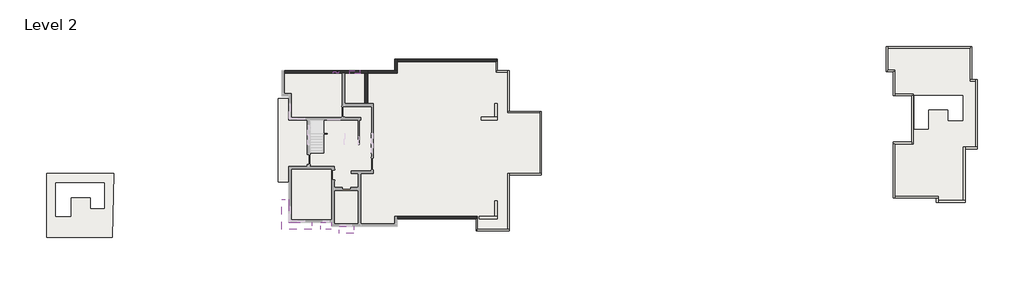
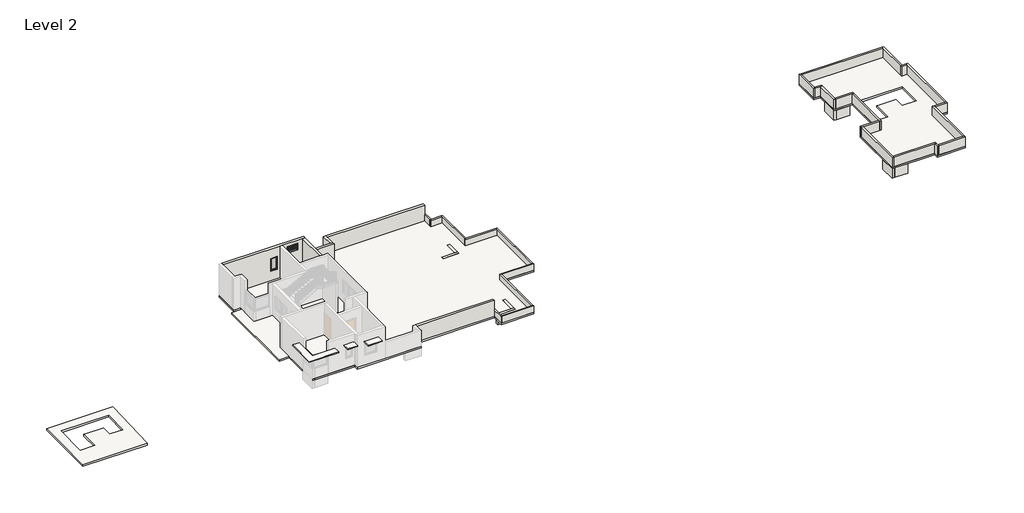
# One storey, part 2 of 5: 39 walls, 4 members, 4 slabs, 2 roofs, 1 plate, 1 window.
"""IFC4 building model written with IfcOpenShell, lengths in millimetres."""

from ifc_helpers import new_model, si_unit, frame, origin, place, context, project, spatial, polyline, outline, extrude, faceted_brep, transform, mapped, element, save
from components import member_75074519, member_86d06fe4, system_panel_glazed_1bcf12e0, window_a18e4be4

model = new_model("IFC4")

# Units and contexts
model_context = context("Model", 3, world=origin())
ifc_project = project(units=[si_unit("LENGTHUNIT", "METRE", prefix="MILLI")], contexts=[model_context])

# Site, building, storey
site = spatial("IfcSite", under=ifc_project)
building = spatial("IfcBuilding", under=site)
storey = spatial("IfcBuildingStorey", under=building, Name="Level 2", Elevation=3048.0)

# Members
placement = place(None, origin())
member_shape = member_75074519(model_context)
element("IfcMember", 1, ObjectType="Rectangular Mullion : 2.5\" x 5\" rectangular", at=placement, inside=storey, context=model_context, shape_type="MappedRepresentation", body=[
    mapped(member_shape, transform((-38334.7146233, 19736.4864709, 3962.4), x_axis=(1.0, 0.0, 0.0), y_axis=(0.0, -1.0, 0.0), z_axis=(0.0, 0.0, -1.0))),
])
element("IfcMember", 2, ObjectType="Rectangular Mullion : 2.5\" x 5\" rectangular", at=placement, inside=storey, context=model_context, shape_type="MappedRepresentation", body=[
    mapped(member_shape, transform((-38944.3146233, 19736.4864709, 5181.6), x_axis=(-1.0, 0.0, 0.0), y_axis=(0.0, -1.0, 0.0), z_axis=(0.0, 0.0, 1.0))),
])
member_2_shape = member_86d06fe4(model_context)
element("IfcMember", 3, ObjectType="Rectangular Mullion : 2.5\" x 5\" rectangular", at=placement, inside=storey, context=model_context, shape_type="MappedRepresentation", body=[
    mapped(member_2_shape, transform((-38398.2146233, 19736.4864709, 5181.6), x_axis=(0.0, 0.0, 1.0), y_axis=(0.0, -1.0, 0.0), z_axis=(1.0, 0.0, 0.0))),
])
element("IfcMember", 4, ObjectType="Rectangular Mullion : 2.5\" x 5\" rectangular", at=placement, inside=storey, context=model_context, shape_type="MappedRepresentation", body=[
    mapped(member_2_shape, transform((-38880.8146233, 19736.4864709, 3962.4), x_axis=(0.0, 0.0, -1.0), y_axis=(0.0, -1.0, 0.0), z_axis=(-1.0, 0.0, 0.0))),
])

# Plate
system_panel_glazed_shape = system_panel_glazed_1bcf12e0(model_context)
element("IfcPlate", 5, ObjectType="System Panel : Glazed", at=placement, inside=storey, context=model_context, shape_type="MappedRepresentation", body=[
    mapped(system_panel_glazed_shape, transform((-38639.5146233, 19736.4864709, 4025.9), x_axis=(1.0, 0.0, 0.0), y_axis=(0.0, 1.0, 0.0), z_axis=(0.0, 0.0, 1.0))),
])

# Roofs
element("IfcRoof", 6, ObjectType="ROOF 6\"", at=placement, inside=storey, context=model_context, shape_type="SweptSolid", body=[
    extrude(outline(polyline([(11387.9100959, 17645.0480703), (11387.9100959, 19778.6480703), (10778.3100959, 19778.6480703), (10778.3100959, 22064.6480703), (18474.5100959, 22064.6480703), (18474.5100959, 19092.8480703), (18969.8100959, 19092.8480703), (18969.8100959, 12844.4480703), (17864.9100959, 12844.4480703), (17864.9100959, 8043.769664), (15274.1100959, 8043.769664), (15274.1100959, 8424.8480703), (11387.9100959, 8424.8480703), (11387.9100959, 13454.0480703), (13064.3100959, 13454.0480703), (13064.3100959, 17645.0480703), (11387.9100959, 17645.0480703)]), holes=[polyline([(17636.3100959, 17645.0480703), (13292.9100959, 17645.0480703), (13292.9100959, 14647.8480703), (14562.9100959, 14647.8480703), (14562.9100959, 16375.0480703), (16366.3100959, 16375.0480703), (16366.3100959, 15409.8480703), (17636.3100959, 15409.8480703), (17636.3100959, 17645.0480703)])]), frame((0.0, 0.0, 3048.0), z_axis=(0.0, 0.0, 1.0), x_axis=(1.0, 0.0, 0.0)), (0.0, 0.0, 1.0), 152.4),
])
element("IfcRoof", 7, ObjectType="ROOF 6\"", at=placement, inside=storey, context=model_context, shape_type="SweptSolid", body=[
    extrude(outline(polyline([(-58617.9939273, 10640.5199577), (-58763.0300618, 4887.4199577), (-64652.8636189, 4887.4199577), (-64652.8636189, 10640.5199577), (-58617.9939273, 10640.5199577)]), holes=[polyline([(-62493.8636189, 6754.3199577), (-62493.8636189, 8481.5199577), (-60690.4636189, 8481.5199577), (-60690.4636189, 7516.3199577), (-59471.2636189, 7516.3199577), (-59471.2636189, 9802.3199577), (-63814.6636189, 9802.3199577), (-63814.6636189, 6754.3199577), (-62493.8636189, 6754.3199577)])]), frame((0.0, 0.0, 3048.0), z_axis=(0.0, 0.0, 1.0), x_axis=(1.0, 0.0, 0.0)), (0.0, 0.0, 1.0), 152.4),
])

# Slabs
element("IfcSlab", 8, ObjectType="FLOOR 6\"", at=placement, inside=storey, context=model_context, shape_type="SweptSolid", body=[
    extrude(outline(polyline([(-43821.1146233, 17357.3026655), (-42906.7146233, 17357.3026655), (-42906.7146233, 17590.1864709), (-43516.3146233, 17590.1864709), (-43516.3146233, 19876.1864709), (-33382.215517, 19876.1864709), (-33382.215517, 20942.9864709), (-24161.5146233, 20942.9864709), (-24161.5146233, 19876.1864709), (-23094.7146233, 19876.1864709), (-23094.7146233, 16218.5864709), (-20199.1146233, 16218.5864709), (-20199.1146233, 10503.5864709), (-23094.7146233, 10503.5864709), (-23094.7146233, 5474.3864709), (-26066.5146233, 5474.3864709), (-26066.5146233, 6541.1864709), (-33153.1146233, 6541.1864709), (-33153.1146233, 5855.3080647), (-39020.5146233, 5855.3080647), (-39020.5146233, 6236.3864709), (-42906.7146233, 6236.3864709), (-42906.7146233, 9893.9864709), (-43821.1146233, 9893.9864709), (-43821.1146233, 17357.3026655)])), frame((0.0, 0.0, 2895.6), z_axis=(0.0, 0.0, 1.0), x_axis=(1.0, 0.0, 0.0)), (0.0, 0.0, 1.0), 152.4),
])
element("IfcSlab", 9, ObjectType="Generic - 12\"", at=placement, inside=storey, context=model_context, shape_type="SweptSolid", body=[
    extrude(outline(polyline([(-43516.3146234, 8293.7864709), (-42906.7146233, 8293.7864709), (-42906.7146233, 6236.3864709), (-40849.3146233, 6236.3864709), (-40849.3146233, 5626.7864709), (-43516.3146234, 5626.7864709), (-43516.3146234, 8293.7864709)])), frame((0.0, 0.0, 5257.8), z_axis=(0.0, 0.0, 1.0), x_axis=(1.0, 0.0, 0.0)), (0.0, 0.0, 1.0), 76.2),
])
element("IfcSlab", 10, ObjectType="Generic - 12\"", at=placement, inside=storey, context=model_context, shape_type="SweptSolid", body=[
    extrude(outline(polyline([(-40011.1146233, 5626.7864709), (-40011.1146233, 6236.3864709), (-39096.7146233, 6236.3864709), (-39096.7146233, 5626.7864709), (-40011.1146233, 5626.7864709)])), frame((0.0, 0.0, 5257.8), z_axis=(0.0, 0.0, 1.0), x_axis=(1.0, 0.0, 0.0)), (0.0, 0.0, 1.0), 76.2),
])
element("IfcSlab", 11, ObjectType="Generic - 12\"", at=placement, inside=storey, context=model_context, shape_type="SweptSolid", body=[
    extrude(outline(polyline([(-38372.8146233, 5245.7080647), (-38372.8146233, 5855.3080647), (-37077.4146233, 5855.3080647), (-37077.4146233, 5245.7080647), (-38372.8146233, 5245.7080647)])), frame((0.0, 0.0, 5257.8), z_axis=(0.0, 0.0, 1.0), x_axis=(1.0, 0.0, 0.0)), (0.0, 0.0, 1.0), 76.2),
])

# Walls
element("IfcWall", 12, at=placement, inside=storey, context=model_context, shape_type="Brep", body=[
    faceted_brep([(-35820.1146233, 19647.5864709, 3048.0), (-33153.615517, 19647.5864709, 3048.0), (-33153.615517, 19647.5864709, 4572.0), (-35820.1146233, 19647.5864709, 4572.0), (-35820.1146233, 19876.1864709, 3048.0), (-35820.1146233, 19876.1864709, 4572.0), (-33382.215517, 19876.1864709, 4572.0), (-33153.615517, 19876.1864709, 4572.0), (-33153.615517, 19876.1864709, 3048.0), (-33382.215517, 19876.1864709, 3048.0)], [[[0, 1, 2, 3]], [[4, 5, 6, 7, 8, 9]], [[1, 0, 4, 9, 8]], [[3, 2, 7, 6, 5]], [[2, 1, 8, 7]], [[0, 3, 5, 4]]]),
])
element("IfcWall", 13, at=placement, inside=storey, context=model_context, shape_type="Brep", body=[
    faceted_brep([(-33153.615517, 19876.1864709, 3048.0), (-33153.615517, 20714.3864709, 3048.0), (-33153.615517, 20942.9864709, 3048.0), (-33153.615517, 20942.9864709, 4572.0), (-33153.615517, 20714.3864709, 4572.0), (-33153.615517, 19876.1864709, 4572.0), (-33382.215517, 19876.1864709, 3048.0), (-33382.215517, 19876.1864709, 4572.0), (-33382.215517, 20942.9864709, 4572.0), (-33382.215517, 20942.9864709, 3048.0)], [[[0, 1, 2, 3, 4, 5]], [[6, 7, 8, 9]], [[2, 1, 0, 6, 9]], [[5, 4, 3, 8, 7]], [[0, 5, 7, 6]], [[3, 2, 9, 8]]]),
])
element("IfcWall", 14, at=placement, inside=storey, context=model_context, shape_type="Brep", body=[
    faceted_brep([(-33153.615517, 20714.3864709, 3048.0), (-24275.8146233, 20714.3864709, 3048.0), (-24275.8146233, 20714.3864709, 4572.0), (-33153.615517, 20714.3864709, 4572.0), (-33153.615517, 20942.9864709, 3048.0), (-33153.615517, 20942.9864709, 4572.0), (-24275.8146233, 20942.9864709, 4572.0), (-24275.8146233, 20942.9864709, 3657.6), (-24275.8146233, 20942.9864709, 3048.0)], [[[0, 1, 2, 3]], [[4, 5, 6, 7, 8]], [[1, 0, 4, 8]], [[3, 2, 6, 5]], [[0, 3, 5, 4]], [[2, 1, 8, 7, 6]]]),
])
element("IfcWall", 15, at=placement, inside=storey, context=model_context, shape_type="Brep", body=[
    faceted_brep([(-33153.1146233, 6541.1864709, 3048.0), (-26066.5146233, 6541.1864709, 3048.0), (-26066.5146233, 6541.1864709, 4572.0), (-33153.1146233, 6541.1864709, 4572.0), (-33153.1146233, 6769.7864709, 3048.0), (-33153.1146233, 6769.7864709, 4572.0), (-26066.5146233, 6769.7864709, 4572.0), (-26066.5146233, 6769.7864709, 3657.6), (-26066.5146233, 6769.7864709, 3048.0)], [[[0, 1, 2, 3]], [[4, 5, 6, 7, 8]], [[1, 0, 4, 8]], [[3, 2, 6, 5]], [[0, 3, 5, 4]], [[2, 1, 8, 7, 6]]]),
])
element("IfcWall", 16, at=placement, inside=storey, context=model_context, shape_type="Brep", body=[
    faceted_brep([(-26066.5146233, 6769.7864709, 3048.0), (-26066.5146233, 6541.1864709, 3048.0), (-26066.5146233, 5474.3864709, 3048.0), (-26066.5146233, 5474.3864709, 3657.6), (-26066.5146233, 6769.7864709, 3657.6), (-25952.2146233, 6769.7864709, 3048.0), (-25952.2146233, 6769.7864709, 3657.6), (-25952.2146233, 5588.6864709, 3657.6), (-25952.2146233, 5474.3864709, 3657.6), (-25952.2146233, 5474.3864709, 3048.0), (-25952.2146233, 5588.6864709, 3048.0)], [[[0, 1, 2, 3, 4]], [[5, 6, 7, 8, 9, 10]], [[2, 1, 0, 5, 10, 9]], [[4, 3, 8, 7, 6]], [[0, 4, 6, 5]], [[3, 2, 9, 8]]]),
])
element("IfcWall", 17, at=placement, inside=storey, context=model_context, shape_type="Brep", body=[
    faceted_brep([(-25952.2146233, 5474.3864709, 3048.0), (-23094.7146233, 5474.3864709, 3048.0), (-23094.7146233, 5474.3864709, 3657.6), (-25952.2146233, 5474.3864709, 3657.6), (-25952.2146233, 5588.6864709, 3048.0), (-25952.2146233, 5588.6864709, 3657.6), (-23209.0146233, 5588.6864709, 3657.6), (-23094.7146233, 5588.6864709, 3657.6), (-23094.7146233, 5588.6864709, 3048.0), (-23209.0146233, 5588.6864709, 3048.0)], [[[0, 1, 2, 3]], [[4, 5, 6, 7, 8, 9]], [[1, 0, 4, 9, 8]], [[3, 2, 7, 6, 5]], [[0, 3, 5, 4]], [[2, 1, 8, 7]]]),
])
element("IfcWall", 18, at=placement, inside=storey, context=model_context, shape_type="Brep", body=[
    faceted_brep([(-23094.7146233, 5588.6864709, 3048.0), (-23094.7146233, 10503.5864709, 3048.0), (-23094.7146233, 10617.8864709, 3048.0), (-23094.7146233, 10617.8864709, 3657.6), (-23094.7146233, 10503.5864709, 3657.6), (-23094.7146233, 5588.6864709, 3657.6), (-23209.0146233, 5588.6864709, 3048.0), (-23209.0146233, 5588.6864709, 3657.6), (-23209.0146233, 10617.8864709, 3657.6), (-23209.0146233, 10617.8864709, 3048.0)], [[[0, 1, 2, 3, 4, 5]], [[6, 7, 8, 9]], [[2, 1, 0, 6, 9]], [[5, 4, 3, 8, 7]], [[0, 5, 7, 6]], [[3, 2, 9, 8]]]),
])
element("IfcWall", 19, at=placement, inside=storey, context=model_context, shape_type="Brep", body=[
    faceted_brep([(-23094.7146233, 10503.5864709, 3048.0), (-20199.1146233, 10503.5864709, 3048.0), (-20199.1146233, 10503.5864709, 3657.6), (-23094.7146233, 10503.5864709, 3657.6), (-23094.7146233, 10617.8864709, 3048.0), (-23094.7146233, 10617.8864709, 3657.6), (-20313.4146233, 10617.8864709, 3657.6), (-20199.1146233, 10617.8864709, 3657.6), (-20199.1146233, 10617.8864709, 3048.0), (-20313.4146233, 10617.8864709, 3048.0)], [[[0, 1, 2, 3]], [[4, 5, 6, 7, 8, 9]], [[1, 0, 4, 9, 8]], [[3, 2, 7, 6, 5]], [[0, 3, 5, 4]], [[2, 1, 8, 7]]]),
])
element("IfcWall", 20, at=placement, inside=storey, context=model_context, shape_type="Brep", body=[
    faceted_brep([(-20199.1146233, 10617.8864709, 3048.0), (-20199.1146233, 16218.5864709, 3048.0), (-20199.1146233, 16218.5864709, 3657.6), (-20199.1146233, 10617.8864709, 3657.6), (-20313.4146233, 10617.8864709, 3048.0), (-20313.4146233, 10617.8864709, 3657.6), (-20313.4146233, 16104.2864709, 3657.6), (-20313.4146233, 16218.5864709, 3657.6), (-20313.4146233, 16218.5864709, 3048.0), (-20313.4146233, 16104.2864709, 3048.0)], [[[0, 1, 2, 3]], [[4, 5, 6, 7, 8, 9]], [[1, 0, 4, 9, 8]], [[3, 2, 7, 6, 5]], [[0, 3, 5, 4]], [[2, 1, 8, 7]]]),
])
element("IfcWall", 21, at=placement, inside=storey, context=model_context, shape_type="Brep", body=[
    faceted_brep([(-20313.4146233, 16218.5864709, 3048.0), (-23094.7146233, 16218.5864709, 3048.0), (-23209.0146233, 16218.5864709, 3048.0), (-23209.0146233, 16218.5864709, 3657.6), (-23094.7146233, 16218.5864709, 3657.6), (-20313.4146233, 16218.5864709, 3657.6), (-20313.4146233, 16104.2864709, 3048.0), (-20313.4146233, 16104.2864709, 3657.6), (-23209.0146233, 16104.2864709, 3657.6), (-23209.0146233, 16104.2864709, 3048.0)], [[[0, 1, 2, 3, 4, 5]], [[6, 7, 8, 9]], [[2, 1, 0, 6, 9]], [[5, 4, 3, 8, 7]], [[0, 5, 7, 6]], [[3, 2, 9, 8]]]),
])
element("IfcWall", 22, at=placement, inside=storey, context=model_context, shape_type="Brep", body=[
    faceted_brep([(-23094.7146233, 16218.5864709, 3048.0), (-23094.7146233, 19876.1864709, 3048.0), (-23094.7146233, 19876.1864709, 3657.6), (-23094.7146233, 16218.5864709, 3657.6), (-23209.0146233, 16218.5864709, 3048.0), (-23209.0146233, 16218.5864709, 3657.6), (-23209.0146233, 19761.8864709, 3657.6), (-23209.0146233, 19876.1864709, 3657.6), (-23209.0146233, 19876.1864709, 3048.0), (-23209.0146233, 19761.8864709, 3048.0)], [[[0, 1, 2, 3]], [[4, 5, 6, 7, 8, 9]], [[1, 0, 4, 9, 8]], [[3, 2, 7, 6, 5]], [[0, 3, 5, 4]], [[2, 1, 8, 7]]]),
])
element("IfcWall", 23, at=placement, inside=storey, context=model_context, shape_type="Brep", body=[
    faceted_brep([(-23209.0146233, 19876.1864709, 3048.0), (-24161.5146233, 19876.1864709, 3048.0), (-24275.8146233, 19876.1864709, 3048.0), (-24275.8146233, 19876.1864709, 3657.6), (-24161.5146233, 19876.1864709, 3657.6), (-23209.0146233, 19876.1864709, 3657.6), (-23209.0146233, 19761.8864709, 3048.0), (-23209.0146233, 19761.8864709, 3657.6), (-24275.8146233, 19761.8864709, 3657.6), (-24275.8146233, 19761.8864709, 3048.0)], [[[0, 1, 2, 3, 4, 5]], [[6, 7, 8, 9]], [[2, 1, 0, 6, 9]], [[5, 4, 3, 8, 7]], [[0, 5, 7, 6]], [[3, 2, 9, 8]]]),
])
element("IfcWall", 24, at=placement, inside=storey, context=model_context, shape_type="Brep", body=[
    faceted_brep([(-24161.5146233, 19876.1864709, 3048.0), (-24161.5146233, 20942.9864709, 3048.0), (-24161.5146233, 20942.9864709, 3657.6), (-24161.5146233, 19876.1864709, 3657.6), (-24275.8146233, 19876.1864709, 3048.0), (-24275.8146233, 19876.1864709, 3657.6), (-24275.8146233, 20942.9864709, 3657.6), (-24275.8146233, 20942.9864709, 3048.0), (-24275.8146233, 20714.3864709, 3048.0)], [[[0, 1, 2, 3]], [[4, 5, 6, 7, 8]], [[1, 0, 4, 8, 7]], [[3, 2, 6, 5]], [[0, 3, 5, 4]], [[2, 1, 7, 6]]]),
])
element("IfcWall", 25, ObjectType="PARAPET WALL", at=placement, inside=storey, context=model_context, shape_type="Brep", body=[
    faceted_brep([(10778.3100959, 22064.6480703, 3200.4), (10778.3100959, 19778.6480703, 3200.4), (10778.3100959, 19778.6480703, 4114.8), (10778.3100959, 22064.6480703, 4114.8), (10930.7100959, 22064.6480703, 3200.4), (10930.7100959, 22064.6480703, 4114.8), (10930.7100959, 21912.2480703, 4114.8), (10930.7100959, 19931.0480703, 4114.8), (10930.7100959, 19778.6480703, 4114.8), (10930.7100959, 19778.6480703, 3200.4), (10930.7100959, 19931.0480703, 3200.4), (10930.7100959, 21912.2480703, 3200.4)], [[[0, 1, 2, 3]], [[4, 5, 6, 7, 8, 9, 10, 11]], [[1, 0, 4, 11, 10, 9]], [[3, 2, 8, 7, 6, 5]], [[2, 1, 9, 8]], [[0, 3, 5, 4]]]),
])
element("IfcWall", 26, ObjectType="PARAPET WALL", at=placement, inside=storey, context=model_context, shape_type="Brep", body=[
    faceted_brep([(10930.7100959, 19778.6480703, 3200.4), (11387.9100959, 19778.6480703, 3200.4), (11540.3100959, 19778.6480703, 3200.4), (11540.3100959, 19778.6480703, 4114.8), (11387.9100959, 19778.6480703, 4114.8), (10930.7100959, 19778.6480703, 4114.8), (10930.7100959, 19931.0480703, 3200.4), (10930.7100959, 19931.0480703, 4114.8), (11540.3100959, 19931.0480703, 4114.8), (11540.3100959, 19931.0480703, 3200.4)], [[[0, 1, 2, 3, 4, 5]], [[6, 7, 8, 9]], [[2, 1, 0, 6, 9]], [[5, 4, 3, 8, 7]], [[0, 5, 7, 6]], [[3, 2, 9, 8]]]),
])
element("IfcWall", 27, ObjectType="PARAPET WALL", at=placement, inside=storey, context=model_context, shape_type="Brep", body=[
    faceted_brep([(11387.9100959, 19778.6480703, 3200.4), (11387.9100959, 17645.0480703, 3200.4), (11387.9100959, 17645.0480703, 4114.8), (11387.9100959, 19778.6480703, 4114.8), (11540.3100959, 19778.6480703, 3200.4), (11540.3100959, 19778.6480703, 4114.8), (11540.3100959, 17797.4480703, 4114.8), (11540.3100959, 17645.0480703, 4114.8), (11540.3100959, 17645.0480703, 3200.4), (11540.3100959, 17797.4480703, 3200.4)], [[[0, 1, 2, 3]], [[4, 5, 6, 7, 8, 9]], [[1, 0, 4, 9, 8]], [[3, 2, 7, 6, 5]], [[0, 3, 5, 4]], [[2, 1, 8, 7]]]),
])
element("IfcWall", 28, ObjectType="PARAPET WALL", at=placement, inside=storey, context=model_context, shape_type="Brep", body=[
    faceted_brep([(11540.3100959, 17645.0480703, 3200.4), (13064.3100959, 17645.0480703, 3200.4), (13216.7100959, 17645.0480703, 3200.4), (13216.7100959, 17645.0480703, 4114.8), (13064.3100959, 17645.0480703, 4114.8), (11540.3100959, 17645.0480703, 4114.8), (11540.3100959, 17797.4480703, 3200.4), (11540.3100959, 17797.4480703, 4114.8), (13216.7100959, 17797.4480703, 4114.8), (13216.7100959, 17797.4480703, 3200.4)], [[[0, 1, 2, 3, 4, 5]], [[6, 7, 8, 9]], [[2, 1, 0, 6, 9]], [[5, 4, 3, 8, 7]], [[0, 5, 7, 6]], [[3, 2, 9, 8]]]),
])
element("IfcWall", 29, ObjectType="PARAPET WALL", at=placement, inside=storey, context=model_context, shape_type="Brep", body=[
    faceted_brep([(13064.3100959, 17645.0480703, 3200.4), (13064.3100959, 13454.0480703, 3200.4), (13064.3100959, 13301.6480703, 3200.4), (13064.3100959, 13301.6480703, 4114.8), (13064.3100959, 13454.0480703, 4114.8), (13064.3100959, 17645.0480703, 4114.8), (13216.7100959, 17645.0480703, 3200.4), (13216.7100959, 17645.0480703, 4114.8), (13216.7100959, 13301.6480703, 4114.8), (13216.7100959, 13301.6480703, 3200.4)], [[[0, 1, 2, 3, 4, 5]], [[6, 7, 8, 9]], [[2, 1, 0, 6, 9]], [[5, 4, 3, 8, 7]], [[0, 5, 7, 6]], [[3, 2, 9, 8]]]),
])
element("IfcWall", 30, ObjectType="PARAPET WALL", at=placement, inside=storey, context=model_context, shape_type="Brep", body=[
    faceted_brep([(13064.3100959, 13454.0480703, 3200.4), (11387.9100959, 13454.0480703, 3200.4), (11387.9100959, 13454.0480703, 4114.8), (13064.3100959, 13454.0480703, 4114.8), (13064.3100959, 13301.6480703, 3200.4), (13064.3100959, 13301.6480703, 4114.8), (11540.3100959, 13301.6480703, 4114.8), (11387.9100959, 13301.6480703, 4114.8), (11387.9100959, 13301.6480703, 3200.4), (11540.3100959, 13301.6480703, 3200.4)], [[[0, 1, 2, 3]], [[4, 5, 6, 7, 8, 9]], [[1, 0, 4, 9, 8]], [[3, 2, 7, 6, 5]], [[0, 3, 5, 4]], [[2, 1, 8, 7]]]),
])
element("IfcWall", 31, ObjectType="PARAPET WALL", at=placement, inside=storey, context=model_context, shape_type="Brep", body=[
    faceted_brep([(11387.9100959, 13301.6480703, 3200.4), (11387.9100959, 8424.8480703, 3200.4), (11387.9100959, 8424.8480703, 4114.8), (11387.9100959, 13301.6480703, 4114.8), (11540.3100959, 13301.6480703, 3200.4), (11540.3100959, 13301.6480703, 4114.8), (11540.3100959, 8577.2480703, 4114.8), (11540.3100959, 8424.8480703, 4114.8), (11540.3100959, 8424.8480703, 3200.4), (11540.3100959, 8577.2480703, 3200.4)], [[[0, 1, 2, 3]], [[4, 5, 6, 7, 8, 9]], [[1, 0, 4, 9, 8]], [[3, 2, 7, 6, 5]], [[0, 3, 5, 4]], [[2, 1, 8, 7]]]),
])
element("IfcWall", 32, ObjectType="PARAPET WALL", at=placement, inside=storey, context=model_context, shape_type="Brep", body=[
    faceted_brep([(11540.3100959, 8424.8480703, 3200.4), (15274.1100959, 8424.8480703, 3200.4), (15426.5100959, 8424.8480703, 3200.4), (15426.5100959, 8424.8480703, 4114.8), (15274.1100959, 8424.8480703, 4114.8), (11540.3100959, 8424.8480703, 4114.8), (11540.3100959, 8577.2480703, 3200.4), (11540.3100959, 8577.2480703, 4114.8), (15426.5100959, 8577.2480703, 4114.8), (15426.5100959, 8577.2480703, 3200.4)], [[[0, 1, 2, 3, 4, 5]], [[6, 7, 8, 9]], [[2, 1, 0, 6, 9]], [[5, 4, 3, 8, 7]], [[0, 5, 7, 6]], [[3, 2, 9, 8]]]),
])
element("IfcWall", 33, ObjectType="PARAPET WALL", at=placement, inside=storey, context=model_context, shape_type="Brep", body=[
    faceted_brep([(15274.1100959, 8424.8480703, 3200.4), (15274.1100959, 8043.769664, 3200.4), (15274.1100959, 8043.769664, 4114.8), (15274.1100959, 8424.8480703, 4114.8), (15426.5100959, 8424.8480703, 3200.4), (15426.5100959, 8424.8480703, 4114.8), (15426.5100959, 8196.169664, 4114.8), (15426.5100959, 8043.769664, 4114.8), (15426.5100959, 8043.769664, 3200.4), (15426.5100959, 8196.169664, 3200.4)], [[[0, 1, 2, 3]], [[4, 5, 6, 7, 8, 9]], [[1, 0, 4, 9, 8]], [[3, 2, 7, 6, 5]], [[0, 3, 5, 4]], [[2, 1, 8, 7]]]),
])
element("IfcWall", 34, ObjectType="PARAPET WALL", at=placement, inside=storey, context=model_context, shape_type="Brep", body=[
    faceted_brep([(15426.5100959, 8043.769664, 3200.4), (17864.9100959, 8043.769664, 3200.4), (17864.9100959, 8043.769664, 4114.8), (15426.5100959, 8043.769664, 4114.8), (15426.5100959, 8196.169664, 3200.4), (15426.5100959, 8196.169664, 4114.8), (17712.5100959, 8196.169664, 4114.8), (17864.9100959, 8196.169664, 4114.8), (17864.9100959, 8196.169664, 3200.4), (17712.5100959, 8196.169664, 3200.4)], [[[0, 1, 2, 3]], [[4, 5, 6, 7, 8, 9]], [[1, 0, 4, 9, 8]], [[3, 2, 7, 6, 5]], [[0, 3, 5, 4]], [[2, 1, 8, 7]]]),
])
element("IfcWall", 35, ObjectType="PARAPET WALL", at=placement, inside=storey, context=model_context, shape_type="Brep", body=[
    faceted_brep([(17864.9100959, 8196.169664, 3200.4), (17864.9100959, 12844.4480703, 3200.4), (17864.9100959, 12996.8480703, 3200.4), (17864.9100959, 12996.8480703, 4114.8), (17864.9100959, 12844.4480703, 4114.8), (17864.9100959, 8196.169664, 4114.8), (17712.5100959, 8196.169664, 3200.4), (17712.5100959, 8196.169664, 4114.8), (17712.5100959, 12996.8480703, 4114.8), (17712.5100959, 12996.8480703, 3200.4)], [[[0, 1, 2, 3, 4, 5]], [[6, 7, 8, 9]], [[2, 1, 0, 6, 9]], [[5, 4, 3, 8, 7]], [[0, 5, 7, 6]], [[3, 2, 9, 8]]]),
])
element("IfcWall", 36, ObjectType="PARAPET WALL", at=placement, inside=storey, context=model_context, shape_type="Brep", body=[
    faceted_brep([(17864.9100959, 12844.4480703, 3200.4), (18969.8100959, 12844.4480703, 3200.4), (18969.8100959, 12844.4480703, 4114.8), (17864.9100959, 12844.4480703, 4114.8), (17864.9100959, 12996.8480703, 3200.4), (17864.9100959, 12996.8480703, 4114.8), (18817.4100959, 12996.8480703, 4114.8), (18969.8100959, 12996.8480703, 4114.8), (18969.8100959, 12996.8480703, 3200.4), (18817.4100959, 12996.8480703, 3200.4)], [[[0, 1, 2, 3]], [[4, 5, 6, 7, 8, 9]], [[1, 0, 4, 9, 8]], [[3, 2, 7, 6, 5]], [[0, 3, 5, 4]], [[2, 1, 8, 7]]]),
])
element("IfcWall", 37, ObjectType="PARAPET WALL", at=placement, inside=storey, context=model_context, shape_type="Brep", body=[
    faceted_brep([(18969.8100959, 12996.8480703, 3200.4), (18969.8100959, 19092.8480703, 3200.4), (18969.8100959, 19092.8480703, 4114.8), (18969.8100959, 12996.8480703, 4114.8), (18817.4100959, 12996.8480703, 3200.4), (18817.4100959, 12996.8480703, 4114.8), (18817.4100959, 18940.4480703, 4114.8), (18817.4100959, 19092.8480703, 4114.8), (18817.4100959, 19092.8480703, 3200.4), (18817.4100959, 18940.4480703, 3200.4)], [[[0, 1, 2, 3]], [[4, 5, 6, 7, 8, 9]], [[1, 0, 4, 9, 8]], [[3, 2, 7, 6, 5]], [[0, 3, 5, 4]], [[2, 1, 8, 7]]]),
])
element("IfcWall", 38, ObjectType="PARAPET WALL", at=placement, inside=storey, context=model_context, shape_type="Brep", body=[
    faceted_brep([(18817.4100959, 19092.8480703, 3200.4), (18474.5100959, 19092.8480703, 3200.4), (18322.1100959, 19092.8480703, 3200.4), (18322.1100959, 19092.8480703, 4114.8), (18474.5100959, 19092.8480703, 4114.8), (18817.4100959, 19092.8480703, 4114.8), (18817.4100959, 18940.4480703, 3200.4), (18817.4100959, 18940.4480703, 4114.8), (18322.1100959, 18940.4480703, 4114.8), (18322.1100959, 18940.4480703, 3200.4)], [[[0, 1, 2, 3, 4, 5]], [[6, 7, 8, 9]], [[2, 1, 0, 6, 9]], [[5, 4, 3, 8, 7]], [[0, 5, 7, 6]], [[3, 2, 9, 8]]]),
])
element("IfcWall", 39, ObjectType="PARAPET WALL", at=placement, inside=storey, context=model_context, shape_type="Brep", body=[
    faceted_brep([(18474.5100959, 19092.8480703, 3200.4), (18474.5100959, 22064.6480703, 3200.4), (18474.5100959, 22064.6480703, 4114.8), (18474.5100959, 19092.8480703, 4114.8), (18322.1100959, 19092.8480703, 3200.4), (18322.1100959, 19092.8480703, 4114.8), (18322.1100959, 21912.2480703, 4114.8), (18322.1100959, 22064.6480703, 4114.8), (18322.1100959, 22064.6480703, 3200.4), (18322.1100959, 21912.2480703, 3200.4)], [[[0, 1, 2, 3]], [[4, 5, 6, 7, 8, 9]], [[1, 0, 4, 9, 8]], [[3, 2, 7, 6, 5]], [[0, 3, 5, 4]], [[2, 1, 8, 7]]]),
])
element("IfcWall", 40, ObjectType="PARAPET WALL", at=placement, inside=storey, context=model_context, shape_type="SweptSolid", body=[
    extrude(outline(polyline([(10930.7100959, 22064.6480703), (18322.1100959, 22064.6480703), (18322.1100959, 21912.2480703), (10930.7100959, 21912.2480703), (10930.7100959, 22064.6480703)])), frame((0.0, 0.0, 3200.4), z_axis=(0.0, 0.0, 1.0), x_axis=(1.0, 0.0, 0.0)), (0.0, 0.0, 1.0), 914.4),
])
element("IfcWall", 41, ObjectType="WALL 9\"", at=placement, inside=storey, context=model_context, shape_type="Brep", body=[
    faceted_brep([(-43287.7146233, 19647.5864709, 3048.0), (-38106.1146233, 19647.5864709, 3048.0), (-37877.5146233, 19647.5864709, 3048.0), (-36048.7146233, 19647.5864709, 3048.0), (-35820.1146233, 19647.5864709, 3048.0), (-35820.1146233, 19647.5864709, 4572.0), (-35820.1146233, 19647.5864709, 6096.0), (-36048.7146233, 19647.5864709, 6096.0), (-37877.5146233, 19647.5864709, 6096.0), (-38106.1146233, 19647.5864709, 6096.0), (-43287.7146233, 19647.5864709, 6096.0), (-38944.3146233, 19647.5864709, 3962.4), (-38944.3146233, 19647.5864709, 5181.6), (-38334.7146233, 19647.5864709, 5181.6), (-38334.7146233, 19647.5864709, 3962.4), (-37420.3146233, 19647.5864709, 5181.6), (-37420.3146233, 19647.5864709, 5791.2), (-36505.9146233, 19647.5864709, 5791.2), (-36505.9146233, 19647.5864709, 5181.6), (-35820.1146233, 19876.1864709, 3048.0), (-43287.7146233, 19876.1864709, 3048.0), (-43287.7146233, 19876.1864709, 6096.0), (-35820.1146233, 19876.1864709, 6096.0), (-35820.1146233, 19876.1864709, 4572.0), (-38944.3146233, 19876.1864709, 5181.6), (-38944.3146233, 19876.1864709, 3962.4), (-38334.7146233, 19876.1864709, 3962.4), (-38334.7146233, 19876.1864709, 5181.6), (-37420.3146233, 19876.1864709, 5791.2), (-37420.3146233, 19876.1864709, 5181.6), (-36505.9146233, 19876.1864709, 5181.6), (-36505.9146233, 19876.1864709, 5791.2)], [[[0, 1, 2, 3, 4, 5, 6, 7, 8, 9, 10], [11, 12, 13, 14], [15, 16, 17, 18]], [[19, 20, 21, 22, 23], [24, 25, 26, 27], [28, 29, 30, 31]], [[4, 3, 2, 1, 0, 20, 19]], [[11, 25, 24, 12]], [[12, 24, 27, 13]], [[13, 27, 26, 14]], [[25, 11, 14, 26]], [[29, 28, 16, 15]], [[30, 29, 15, 18]], [[31, 30, 18, 17]], [[28, 31, 17, 16]], [[10, 9, 8, 7, 6, 22, 21]], [[4, 19, 23, 22, 6, 5]], [[0, 10, 21, 20]]]),
])
element("IfcWall", 42, ObjectType="WALL 9\"", at=placement, inside=storey, context=model_context, shape_type="SweptSolid", body=[
    extrude(outline(polyline([(-36048.7146233, 16904.3864709), (-36048.7146233, 19647.5864709), (-35820.1146233, 19647.5864709), (-35820.1146233, 16904.3864709), (-36048.7146233, 16904.3864709)])), frame((0.0, 0.0, 3048.0), z_axis=(0.0, 0.0, 1.0), x_axis=(1.0, 0.0, 0.0)), (0.0, 0.0, 1.0), 3048.0),
])
element("IfcWall", 43, ObjectType="WALL 9\" 2", at=placement, inside=storey, context=model_context, shape_type="Brep", body=[
    faceted_brep([(11387.9100959, 9872.649831, 2133.6), (11387.9100959, 8424.8480703, 2133.6), (11387.9100959, 8424.8480703, 3048.0), (11387.9100959, 9872.649831, 3048.0), (11616.5100959, 9872.649831, 2133.6), (11616.5100959, 9872.649831, 3048.0), (11616.5100959, 8653.4480703, 3048.0), (11616.5100959, 8424.8480703, 3048.0), (11616.5100959, 8424.8480703, 2133.6), (11616.5100959, 8653.4480703, 2133.6)], [[[0, 1, 2, 3]], [[4, 5, 6, 7, 8, 9]], [[1, 0, 4, 9, 8]], [[0, 3, 5, 4]], [[2, 1, 8, 7]], [[3, 2, 7, 6, 5]]]),
])
element("IfcWall", 44, ObjectType="WALL 9\" 2", at=placement, inside=storey, context=model_context, shape_type="SweptSolid", body=[
    extrude(outline(polyline([(12835.7100959, 8424.8480703), (11616.5100959, 8424.8480703), (11616.5100959, 8653.4480703), (12835.7100959, 8653.4480703), (12835.7100959, 8424.8480703)])), frame((0.0, 0.0, 2133.6), z_axis=(0.0, 0.0, 1.0), x_axis=(1.0, 0.0, 0.0)), (0.0, 0.0, 1.0), 914.4),
])
element("IfcWall", 45, ObjectType="WALL 9\" 2", at=placement, inside=storey, context=model_context, shape_type="Brep", body=[
    faceted_brep([(11387.9100959, 19092.8480703, 2133.6), (11387.9100959, 17645.0480703, 2133.6), (11387.9100959, 17645.0480703, 3048.0), (11387.9100959, 19092.8480703, 3048.0), (11616.5100959, 19092.8480703, 2133.6), (11616.5100959, 19092.8480703, 3048.0), (11616.5100959, 17873.6480703, 3048.0), (11616.5100959, 17645.0480703, 3048.0), (11616.5100959, 17645.0480703, 2133.6), (11616.5100959, 17873.6480703, 2133.6)], [[[0, 1, 2, 3]], [[4, 5, 6, 7, 8, 9]], [[1, 0, 4, 9, 8]], [[0, 3, 5, 4]], [[2, 1, 8, 7]], [[3, 2, 7, 6, 5]]]),
])
element("IfcWall", 46, ObjectType="WALL 9\" 2", at=placement, inside=storey, context=model_context, shape_type="SweptSolid", body=[
    extrude(outline(polyline([(12835.7100959, 17645.0480703), (11616.5100959, 17645.0480703), (11616.5100959, 17873.6480703), (12835.7100959, 17873.6480703), (12835.7100959, 17645.0480703)])), frame((0.0, 0.0, 2133.6), z_axis=(0.0, 0.0, 1.0), x_axis=(1.0, 0.0, 0.0)), (0.0, 0.0, 1.0), 914.4),
])
element("IfcWall", 47, ObjectType="wall 3'", at=placement, inside=storey, context=model_context, shape_type="Brep", body=[
    faceted_brep([(-25761.7146233, 6547.9624892, 2133.6), (-24161.5146233, 6547.9624892, 2133.6), (-24161.5146233, 6547.9624892, 3048.0), (-25761.7146233, 6547.9624892, 3048.0), (-25761.7146233, 6776.5624892, 2133.6), (-25761.7146233, 6776.5624892, 3048.0), (-24390.1146233, 6776.5624892, 3048.0), (-24161.5146233, 6776.5624892, 3048.0), (-24161.5146233, 6776.5624892, 2133.6), (-24390.1146233, 6776.5624892, 2133.6)], [[[0, 1, 2, 3]], [[4, 5, 6, 7, 8, 9]], [[1, 0, 4, 9, 8]], [[3, 2, 7, 6, 5]], [[0, 3, 5, 4]], [[2, 1, 8, 7]]]),
])
element("IfcWall", 48, ObjectType="wall 3'", at=placement, inside=storey, context=model_context, shape_type="SweptSolid", body=[
    extrude(outline(polyline([(-24161.5146233, 8148.1624892), (-24161.5146233, 6776.5624892), (-24390.1146233, 6776.5624892), (-24390.1146233, 8148.1624892), (-24161.5146233, 8148.1624892)])), frame((0.0, 0.0, 2133.6), z_axis=(0.0, 0.0, 1.0), x_axis=(1.0, 0.0, 0.0)), (0.0, 0.0, 1.0), 914.4),
])
element("IfcWall", 49, ObjectType="wall 3'", at=placement, inside=storey, context=model_context, shape_type="Brep", body=[
    faceted_brep([(-25609.3146233, 15463.3624892, 2133.6), (-24161.5146233, 15463.3624892, 2133.6), (-24161.5146233, 15463.3624892, 3048.0), (-25609.3146233, 15463.3624892, 3048.0), (-25609.3146233, 15691.9624892, 2133.6), (-25609.3146233, 15691.9624892, 3048.0), (-24390.1146233, 15691.9624892, 3048.0), (-24161.5146233, 15691.9624892, 3048.0), (-24161.5146233, 15691.9624892, 2133.6), (-24390.1146233, 15691.9624892, 2133.6)], [[[0, 1, 2, 3]], [[4, 5, 6, 7, 8, 9]], [[1, 0, 4, 9, 8]], [[3, 2, 7, 6, 5]], [[0, 3, 5, 4]], [[2, 1, 8, 7]]]),
])
element("IfcWall", 50, ObjectType="wall 3'", at=placement, inside=storey, context=model_context, shape_type="SweptSolid", body=[
    extrude(outline(polyline([(-24161.5146233, 16911.1624892), (-24161.5146233, 15691.9624892), (-24390.1146233, 15691.9624892), (-24390.1146233, 16911.1624892), (-24161.5146233, 16911.1624892)])), frame((0.0, 0.0, 2133.6), z_axis=(0.0, 0.0, 1.0), x_axis=(1.0, 0.0, 0.0)), (0.0, 0.0, 1.0), 914.4),
])

# Window
window_shape = window_a18e4be4(model_context)
element("IfcWindow", 51, ObjectType="Window-Louvers : 36\" x 24\"", at=placement, inside=storey, context=model_context, shape_type="MappedRepresentation", body=[
    mapped(window_shape, transform((-36963.1146233, 19768.2364709, 4267.2), x_axis=(1.0, 0.0, 0.0), y_axis=(0.0, 1.0, 0.0), z_axis=(0.0, 0.0, 1.0))),
])

save(model, "model.ifc")

# Revit data of these elements
# Type "Rectangular Mullion : 2.5\" x 5\" rectangular"
#   built-in parameter 1007304 = 0.416667 (stored number, unit not read)
#   built-in parameter 1007301 = 0.104167 (stored number, unit not read)
#   built-in parameter 1007300 = 0.104167 (stored number, unit not read)
# Type "System Panel : Glazed"
#   Construction Type Id = "GSP4R"
#   Analytic Construction = "1/8 in Pilkington single glazing"
#   Visual Light Transmittance = 0.9
#   Solar Heat Gain Coefficient = 0.86
#   Heat Transfer Coefficient (U) = 1.18115 BTU/(h·ft²·°F)
#   Define Thermal Properties by = 1
# Type "ROOF 6\""
#   Assembly Code = "B1020"
#   Layers, outside or top first: 0' - 6" no material (function 1)
# Type "FLOOR 6\""
#   Assembly Code = "B1010"
#   Function = 0
#   Layers, outside or top first: 0' - 6" no material (function 1)
# Type "Generic - 12\""
#   Assembly Code = "B1010"
#   Function = 0
#   Layers, outside or top first: 0' - 3" no material (function 1)
# Type
#   Assembly Code = "B2010"
#   Layers, outside or top first: 0' - 9" no material (function 1)
# Type
#   Assembly Code = "B2010"
#   Layers, outside or top first: 0' - 4 1/2" no material (function 1)
# Type "PARAPET WALL"
#   Assembly Code = "B2010"
#   Layers, outside or top first: 0' - 6" no material (function 1)
# Type "WALL 9\""
#   Assembly Code = "B2010"
#   Layers, outside or top first: 0' - 9" no material (function 1)
# Type "WALL 9\" 2"
#   Assembly Code = "B2010"
#   Layers, outside or top first: 0' - 9" no material (function 1)
# Type "wall 3'"
#   Assembly Code = "B2010"
#   Layers, outside or top first: 0' - 9" no material (function 1)
# Type "Window-Louvers : 36\" x 24\""
#   Type Mark = "18"
#   Construction Type Id = "GSP4R"
#   Assembly Code = "B20"
#   Analytic Construction = "1/8 in Pilkington single glazing"
#   Visual Light Transmittance = 0.9
#   Thermal Resistance (R) = 1.53941 (h·ft²·°F)/BTU
#   Solar Heat Gain Coefficient = 0.78
#   Max Height = 1' - 11.74264"
#   Height = 2' - 0"
#   Heat Transfer Coefficient (U) = 0.6496 BTU/(h·ft²·°F)
#   Blade Width [instance default] = 2' - 10 1/2"
#   Blade Vertical Thickness = 0' - 0.35355"
#   Blade Thickness = 0' - 0 1/4"
#   Blade Spacing = 0' - 1 1/2"
#   Blade Height = 0' - 1.85355"
#   Blade Depth = 0' - 3"
#   Blade Angle = 45.00°
#   Default Sill Height = 3' - 0"
#   Trim Projection_Exterior = 0' - 0 1/2"
#   Trim Projection_Interior = 0' - 0 1/2"
#   Trim Width_Exterior = 0' - 1 1/2"
#   Trim Width_Interior = 0' - 1 1/2"
#   Width = 3' - 0"
#   Max Blade Count = 12
#   Define Thermal Properties by = 1
#   Blade Count = 12
#   Frame Material = Birch
#   Louver Material = Birch
#   Trim Exterior Material = Birch
#   Trim Interior Material = Birch
#   Wall Closure = (empty or 0)
# Elements 1, 2, 3, 4 (IfcMember, "Rectangular Mullion : 2.5\" x 5\" rectangular")
#   Phase Created = New Construction
#   Materials on its faces: "Aluminum"
# Element 5 (IfcPlate, "System Panel : Glazed")
#   Phase Created = New Construction
#   Materials on its faces: "Glass"
# Elements 6, 7 (IfcRoof, "ROOF 6\"")
#   built-in parameter 1001705 = 10.5 (stored number, unit not read)
#   built-in parameter 1001710 = 33615
#   Phase Created = New Construction
#   Materials on its faces: "Default Roof"
# Element 8 (IfcSlab, "FLOOR 6\"")
#   built-in parameter 1001955 = 3.14159 (stored number, unit not read)
#   Height Offset From Level = 0' - 0"
#   Phase Created = New Construction
#   Materials on its faces: "Copper", "Default Floor", "Wood Planks"
# Element 9 (IfcSlab, "Generic - 12\"")
#   built-in parameter 1001955 = 3.14159 (stored number, unit not read)
#   Height Offset From Level = 7' - 6"
#   Phase Created = New Construction
#   Materials on its faces: "Parking Stripe", "Default Floor"
# Element 10 (IfcSlab, "Generic - 12\"")
#   built-in parameter 1001955 = -1.5708 (stored number, unit not read)
#   Height Offset From Level = 7' - 6"
#   Phase Created = New Construction
#   Materials on its faces: "Parking Stripe", "Default Floor"
# Element 11 (IfcSlab, "Generic - 12\"")
#   built-in parameter 1001955 = -1.5708 (stored number, unit not read)
#   Height Offset From Level = 7' - 6"
#   Phase Created = New Construction
#   Materials on its faces: "Default Floor", "Parking Stripe"
# Elements 12, 13, 14 (IfcWall)
#   Top Offset = 0' - 0"
#   Base Offset = 0' - 0"
#   Unconnected Height = 5' - 0"
#   wall height = 5' - 0"
#   Phase Created = New Construction
#   Base Constraint = Level 2
#   Materials on its faces: "Clad - White", "Default Wall", "Copper"
# Element 15 (IfcWall)
#   Top Offset = 0' - 0"
#   Base Offset = 0' - 0"
#   Unconnected Height = 5' - 0"
#   wall height = 5' - 0"
#   Phase Created = New Construction
#   Base Constraint = Level 2
#   Materials on its faces: "Default Wall", "Clad - White", "Copper"
# Elements 16, 19 (IfcWall)
#   Top Offset = 0' - 0"
#   Base Offset = 0' - 0"
#   Unconnected Height = 2' - 0"
#   wall height = 2' - 0"
#   Phase Created = New Construction
#   Base Constraint = Level 2
#   Materials on its faces: "Clad - White", "Default Wall"
# Elements 17, 18, 20, 21, 22, 23, 24 (IfcWall)
#   Top Offset = 0' - 0"
#   Base Offset = 0' - 0"
#   Unconnected Height = 2' - 0"
#   wall height = 2' - 0"
#   Phase Created = New Construction
#   Base Constraint = Level 2
#   Materials on its faces: "Clad - White", "Default Wall", "Copper"
# Elements 25, 26, 27, 28, 29, 30, 31, 32, 33, 34, 35, 36, 37, 38, 39, 40 (IfcWall, "PARAPET WALL")
#   built-in parameter 1001111 = 0' - 6"
#   Top Offset = 0' - 0"
#   Base Offset = 0' - 6"
#   Unconnected Height = 3' - 0"
#   wall height = 3' - 0"
#   Phase Created = New Construction
#   Base Constraint = Level 2
#   Materials on its faces: "Default Wall"
# Elements 41, 42 (IfcWall, "WALL 9\"")
#   Top Offset = 0' - 0"
#   Base Offset = 0' - 0"
#   Unconnected Height = 10' - 0"
#   wall height = 10' - 0"
#   Phase Created = New Construction
#   Base Constraint = Level 2
#   Materials on its faces: "Default Wall", "Wood Planks"
# Elements 43, 44, 45, 46 (IfcWall, "WALL 9\" 2")
#   built-in parameter 1001111 = -3' - 0"
#   Top Offset = 0' - 0"
#   Base Offset = -3' - 0"
#   Unconnected Height = 3' - 0"
#   wall height = 3' - 0"
#   Phase Created = New Construction
#   Base Constraint = Level 2
#   Materials on its faces: "Default Wall"
# Elements 47, 48, 49, 50 (IfcWall, "wall 3'")
#   built-in parameter 1001111 = -3' - 0"
#   Top Offset = 0' - 0"
#   Base Offset = -3' - 0"
#   Unconnected Height = 3' - 0"
#   wall height = 3' - 0"
#   Phase Created = New Construction
#   Base Constraint = Level 2
#   Materials on its faces: "Default Wall", "Wood Planks"
# Element 51 (IfcWindow, "Window-Louvers : 36\" x 24\"")
#   Mark = "7"
#   Blade Width = 2' - 10 1/2"
#   Phase Created = New Construction
#   Materials on its faces: "Birch"
# Materials
#   "Birch": class "Wood", colour RGB 224 178 126, transparency 0, Description = "Betula Alleghaniensis", Cost = 0
#   "Aluminum": class "Metal", colour RGB 247 247 247, transparency 0, Description = "Aluminum 6061", Cost = 0
#   "Glass": class "Glass", colour RGB 0 128 192, transparency 0.75, Description = "Soda Lime Glass", Cost = 0
#   "Default Roof": colour RGB 88 101 114, transparency 0, Cost = 0
#   "Copper": class "Metal", colour RGB 0 0 0, transparency 0, Description = "Copper, matte finish", Cost = 0
#   "Default Floor": colour RGB 128 128 128, transparency 0, Cost = 0
#   "Wood Planks": class "Wood", colour RGB 193 160 115, transparency 0, Description = "Physical material.", Cost = 0
#   "Parking Stripe": class "Paint", colour RGB 250 250 91, transparency 0, Cost = 0
#   "Clad - White": class "Wood", colour RGB 242 242 238, transparency 0, Cost = 0
#   "Default Wall": colour RGB 128 128 128, transparency 0, Cost = 0
